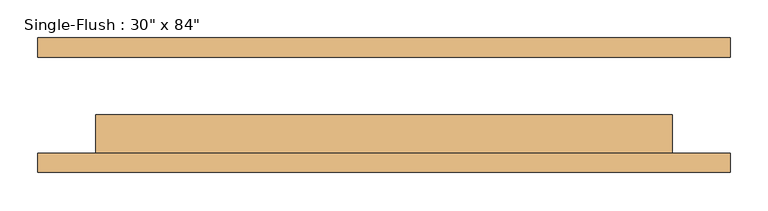
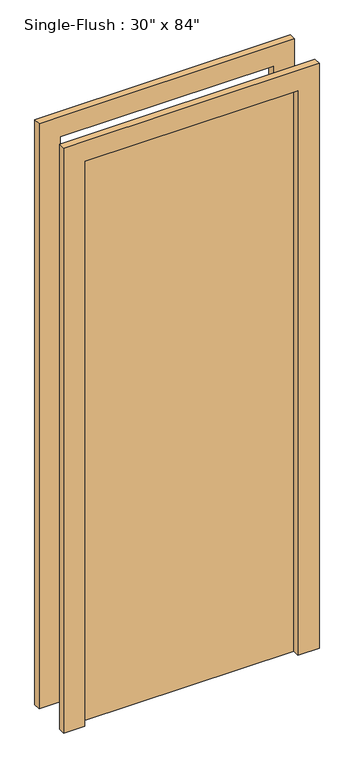
"""IFC4 building model written with IfcOpenShell, lengths in millimetres: door geometry."""

from ifc_helpers import new_model, si_unit, frame, origin, origin_with_axes, place, context, project, spatial, polyline, outline, extrude, source, transform, mapped, element, save


def door_e36758a9(model_context):
    return source(origin(), model_context, "Body", "SweptSolid", [
        extrude(outline(polyline([(2209.8, -457.2), (0.0, -457.2), (0.0, -381.0), (2133.6, -381.0), (2133.6, 381.0), (0.0, 381.0), (0.0, 457.2), (2209.8, 457.2), (2209.8, -457.2)])), frame((0.0, -88.9, 0.0), z_axis=(0.0, 1.0, 0.0), x_axis=(0.0, 0.0, 1.0)), (0.0, 0.0, 1.0), 25.4),
        extrude(outline(polyline([(2209.8, 457.2), (2209.8, -457.2), (0.0, -457.2), (0.0, -381.0), (2133.6, -381.0), (2133.6, 381.0), (0.0, 381.0), (0.0, 457.2), (2209.8, 457.2)])), frame((0.0, 63.5, 0.0), z_axis=(0.0, 1.0, 0.0), x_axis=(0.0, 0.0, 1.0)), (0.0, 0.0, 1.0), 25.4),
        extrude(outline(polyline([(381.0, -12.7), (381.0, -63.5), (-381.0, -63.5), (-381.0, -12.7), (381.0, -12.7)])), origin_with_axes(), (0.0, 0.0, 1.0), 2133.6),
    ])


if __name__ == "__main__":
    model = new_model("IFC4")
    model_context = context("Model", 3, world=origin())
    ifc_project = project(units=[si_unit("LENGTHUNIT", "METRE", prefix="MILLI")], contexts=[model_context])
    site = spatial("IfcSite", under=ifc_project)
    building = spatial("IfcBuilding", under=site)
    placement = place(None, origin())
    door_shape = door_e36758a9(model_context)
    element("IfcDoor", 1, ObjectType="Single-Flush : 30\" x 84\"", at=placement, inside=building, context=model_context, shape_type="MappedRepresentation", body=[
        mapped(door_shape, transform((0.0, 0.0, 0.0), x_axis=(1.0, 0.0, 0.0), y_axis=(0.0, 1.0, 0.0), z_axis=(0.0, 0.0, 1.0))),
    ])
    save(model, "model.ifc")

# Revit data of these elements
# Type "Single-Flush : 30\" x 84\""
#   Type Mark = "4"
#   Construction Type Id = "MDOOR"
#   Assembly Code = "C1020"
#   Analytic Construction = "Metal"
#   Thickness = 0' - 2"
#   Heat Transfer Coefficient (U) = 0.651978 BTU/(h·ft²·°F)
#   Height = 7' - 0"
#   Trim Projection Ext = 0' - 1"
#   Trim Projection Int = 0' - 1"
#   Trim Width = 0' - 3"
#   Width = 2' - 6"
#   Define Thermal Properties by = 1
#   Define Thermal Properties by = 1
#   Door Material = Door - Panel
#   Frame Material = Door - Frame
#   Visual Light Transmittance = 0
#   Solar Heat Gain Coefficient = 0
#   Function = (empty or 0)
#   Wall Closure = (empty or 0)
# Element 1 (IfcDoor, "Single-Flush : 30\" x 84\"")
#   Materials on its faces: "Door - Frame", "Door - Panel"
# Materials
#   "Door - Panel": class "Wood", colour RGB 210 159 95, transparency 0, Cost = 0
#   "Door - Frame": colour RGB 118 70 51, transparency 0, Cost = 0
